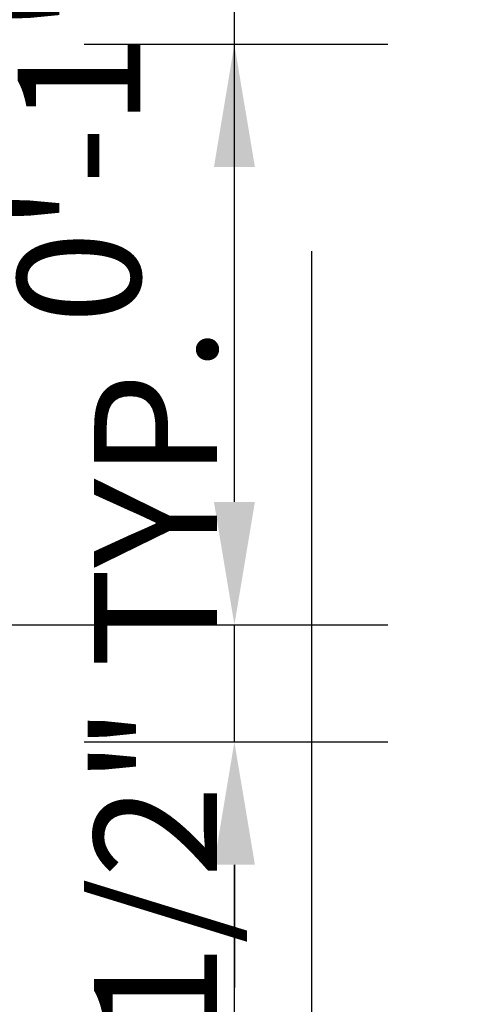
# Model space of a CAD drawing. Units: millimetres. Extents: x 7894 to 8038, y 6851 to 6951.
# Tile 13 of 49: x 7980.935 to 7984.563, y 6870.767 to 6878.784. Entities that reach past the tile are written whole.
import ezdxf

# ---------------------------------------------------------------- set-up
doc = ezdxf.new("R2010")
doc.units = ezdxf.units.MM
doc.layers.add('A-ANNO-DIMS', color=2, linetype='Continuous', lineweight=18)
doc.styles.get("Standard").update_dxf_attribs({"font": 'arial.ttf'})
doc.dimstyles.new('ISO-25', dxfattribs={"dimtxt": 1, "dimasz": 1, "dimexe": 1.25, "dimexo": 0.625, "dimtad": 1, "dimdec": 0, "dimlunit": 4, "dimtxsty": 'Standard', "dimcen": 2.5, "dimclrt": 1, "dimadec": 0, "dimazin": 0, "dimtfac": 1, "dimtdec": 0, "dimtmove": 0, "dimatfit": 3, "dimfxl": 1, "dimarcsym": 0})

# ---------------------------------------------------------------- blocks, each defined once
blk = doc.blocks.new('*D22')
at = {"layer": 'A-ANNO-DIMS', "color": 0, "lineweight": -2, "transparency": 16777216}
for p, q in [((7983.3131, 6866.2225), (7983.3131, 6876.8981)), ((7981.3426, 6865.2225), (7984.5631, 6865.2225)), ((7983.3131, 6864.7225), (7983.3131, 6865.2225)), ((7981.3426, 6864.7225), (7984.5631, 6864.7225)), ((7983.3131, 6863.7225), (7983.3131, 6862.7225))]:
    blk.add_line(p, q, dxfattribs=at)
at = {"layer": 'A-ANNO-DIMS', "color": 0, "transparency": 16777216}
for points in [[(7983.1464, 6866.2225), (7983.4798, 6866.2225), (7983.3131, 6865.2225)], [(7983.1464, 6863.7225), (7983.4798, 6863.7225), (7983.3131, 6864.7225)]]:
    blk.add_solid(points, dxfattribs=at)
at = {"layer": 'Defpoints', "color": 0, "transparency": 16777216}
for p in [(7980.7176, 6865.2225), (7983.3131, 6865.2225), (7980.7176, 6864.7225)]:
    blk.add_point(p, dxfattribs=at)
at = {"layer": 'A-ANNO-DIMS', "color": 1, "transparency": 16777216, "insert": (7982.171, 6872.0603), "char_height": 1, "attachment_point": 5, "rotation": 90}
blk.add_mtext('0\'-0 1/2" TYP.', dxfattribs=at)
blk = doc.blocks.new('*D38')
at = {"layer": 'A-ANNO-DIMS', "color": 0, "lineweight": -2, "transparency": 16777216}
for p, q in [((7981.4609, 6872.9028), (7983.9334, 6872.9028)), ((7982.6834, 6865.7225), (7982.6834, 6871.9028)), ((7981.3426, 6864.7225), (7983.9334, 6864.7225))]:
    blk.add_line(p, q, dxfattribs=at)
at = {"layer": 'A-ANNO-DIMS', "color": 0, "transparency": 16777216}
for points in [[(7982.5168, 6871.9028), (7982.8501, 6871.9028), (7982.6834, 6872.9028)], [(7982.5168, 6865.7225), (7982.8501, 6865.7225), (7982.6834, 6864.7225)]]:
    blk.add_solid(points, dxfattribs=at)
at = {"layer": 'Defpoints', "color": 0, "transparency": 16777216}
for p in [(7980.8359, 6872.9028), (7982.6834, 6872.9028), (7980.7176, 6864.7225)]:
    blk.add_point(p, dxfattribs=at)
at = {"layer": 'A-ANNO-DIMS', "color": 1, "transparency": 16777216, "insert": (7981.5479, 6868.8127), "char_height": 1, "attachment_point": 5, "rotation": 90}
blk.add_mtext('0\'-8"', dxfattribs=at)
blk = doc.blocks.new('*D39')
at = {"layer": 'A-ANNO-DIMS', "color": 0, "lineweight": -2, "transparency": 16777216}
for p, q in [((7982.6834, 6874.8578), (7982.6834, 6879.7661)), ((7964.1574, 6873.8578), (7983.9334, 6873.8578)), ((7982.6834, 6872.9028), (7982.6834, 6873.8578)), ((7981.4609, 6872.9028), (7983.9334, 6872.9028)), ((7982.6834, 6871.9028), (7982.6834, 6870.9028))]:
    blk.add_line(p, q, dxfattribs=at)
at = {"layer": 'A-ANNO-DIMS', "color": 0, "transparency": 16777216}
for points in [[(7982.5168, 6874.8578), (7982.8501, 6874.8578), (7982.6834, 6873.8578)], [(7982.5168, 6871.9028), (7982.8501, 6871.9028), (7982.6834, 6872.9028)]]:
    blk.add_solid(points, dxfattribs=at)
at = {"layer": 'Defpoints', "color": 0, "transparency": 16777216}
for p in [(7963.5324, 6873.8578), (7982.6834, 6873.8578), (7980.8359, 6872.9028)]:
    blk.add_point(p, dxfattribs=at)
at = {"layer": 'A-ANNO-DIMS', "color": 1, "transparency": 16777216, "insert": (7981.5479, 6877.8119), "char_height": 1, "attachment_point": 5, "rotation": 90}
blk.add_mtext('0\'-1"', dxfattribs=at)
blk = doc.blocks.new('*D40')
at = {"layer": 'A-ANNO-DIMS', "color": 0, "lineweight": -2, "transparency": 16777216}
for p, q in [((7982.6834, 6878.5836), (7982.6834, 6885.822)), ((7981.4609, 6878.5836), (7983.9334, 6878.5836)), ((7982.6834, 6874.8578), (7982.6834, 6877.5836)), ((7964.1574, 6873.8578), (7983.9334, 6873.8578))]:
    blk.add_line(p, q, dxfattribs=at)
at = {"layer": 'A-ANNO-DIMS', "color": 0, "transparency": 16777216}
for points in [[(7982.5168, 6877.5836), (7982.8501, 6877.5836), (7982.6834, 6878.5836)], [(7982.5168, 6874.8578), (7982.8501, 6874.8578), (7982.6834, 6873.8578)]]:
    blk.add_solid(points, dxfattribs=at)
at = {"layer": 'Defpoints', "color": 0, "transparency": 16777216}
for p in [(7980.8359, 6878.5836), (7982.6834, 6878.5836), (7963.5324, 6873.8578)]:
    blk.add_point(p, dxfattribs=at)
at = {"layer": 'A-ANNO-DIMS', "color": 1, "transparency": 16777216, "insert": (7981.5414, 6882.7028), "char_height": 1, "attachment_point": 5, "rotation": 90}
blk.add_mtext('0\'-4 1/2"', dxfattribs=at)

msp = doc.modelspace()

# ---------------------------------------------------------------- dimensions: what is measured, and where the dimension line sits
at = {"layer": 'A-ANNO-DIMS'}
for base, p1, p2, picture, middle in [((7982.6834, 6878.5836), (7963.5324, 6873.8578), (7980.8359, 6878.5836), '*D40', (7981.5414, 6882.7028)), ((7982.6834, 6873.8578), (7980.8359, 6872.9028), (7963.5324, 6873.8578), '*D39', (7981.5479, 6877.8119)), ((7982.6834, 6872.9028), (7980.7176, 6864.7225), (7980.8359, 6872.9028), '*D38', (7981.5479, 6868.8127))]:
    dim = msp.add_linear_dim(base=base, p1=p1, p2=p2, angle=90, dimstyle='ISO-25', override={"dimdec": 1, "dimlfac": 1, "dimrnd": 0, "dimzin": 1, "dimdsep": 46, "dimlunit": 4, "dimfrac": 2}, dxfattribs=at)
    dim.commit()
    dim.dimension.update_dxf_attribs({"geometry": picture, "text_midpoint": middle})
dim = msp.add_linear_dim(base=(7983.3131, 6865.2225), p1=(7980.7176, 6864.7225), p2=(7980.7176, 6865.2225), angle=90, text='<> TYP.', dimstyle='ISO-25', override={"dimdec": 1, "dimlfac": 1, "dimrnd": 0, "dimzin": 1, "dimdsep": 46, "dimlunit": 4, "dimfrac": 2}, dxfattribs=at)
dim.commit()
dim.dimension.update_dxf_attribs({"geometry": '*D22', "text_midpoint": (7982.171, 6872.0603)})

doc.saveas('drawing.dxf')
